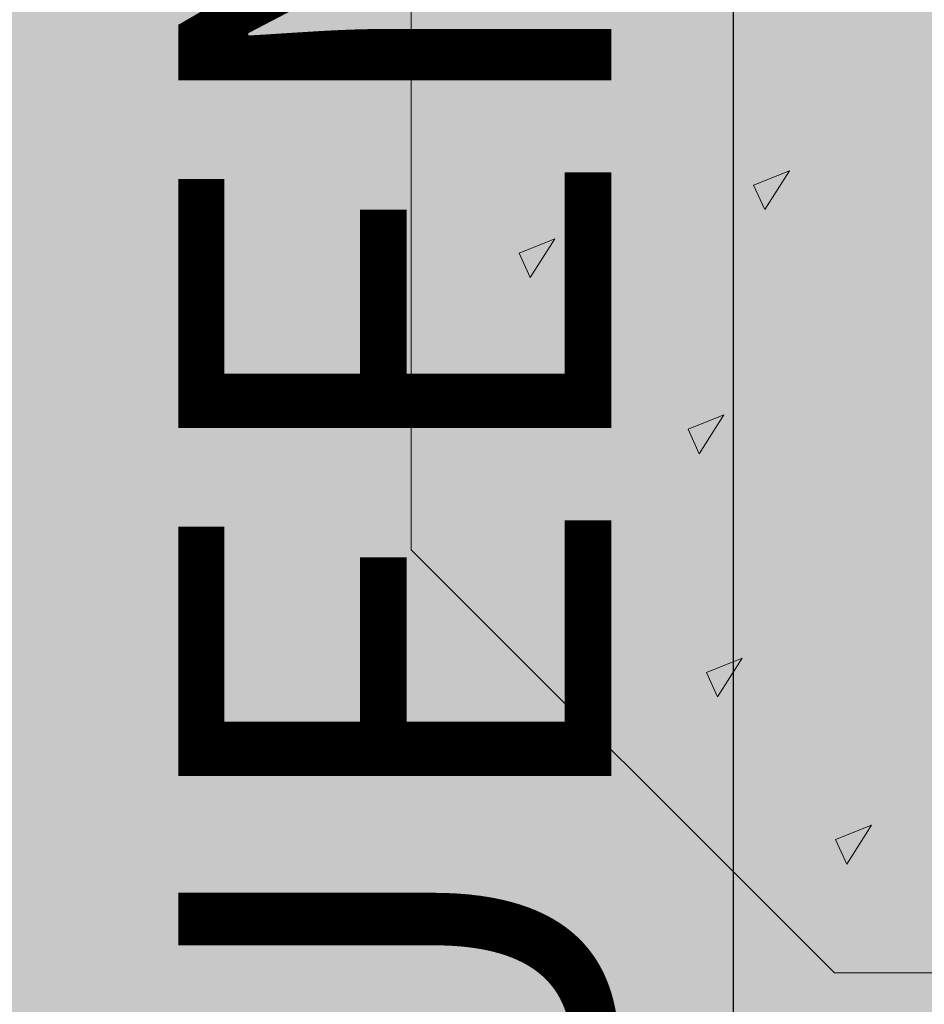
# Model space of a CAD drawing. Units: inches. Extents: x 459864 to 460310, y 324185 to 324787.
# Tile 46 of 112: x 460127.39 to 460139.92, y 324211.25 to 324224.9. Entities that reach past the tile are written whole.
import ezdxf

# ---------------------------------------------------------------- set-up
doc = ezdxf.new("R2010")
doc.units = ezdxf.units.IN
for name, color, linetype, lineweight in [('A-ANNO-DIMS', 2, 'Continuous', 18), ('L-HRDS', 9, 'Continuous', 18), ('L-SITE-PATT', 252, 'Continuous', 13)]:
    doc.layers.add(name, color=color, linetype=linetype, lineweight=lineweight)
doc.styles.get("Standard").update_dxf_attribs({"font": 'arial.ttf'})
doc.dimstyles.new('ISO-25', dxfattribs={"dimtxt": 6, "dimasz": 2.5, "dimexe": 1.25, "dimexo": 0.625, "dimtad": 1, "dimdec": 1, "dimlunit": 3, "dimtxsty": 'Standard', "dimcen": 2.5, "dimadec": 0, "dimazin": 0, "dimtfac": 1, "dimtdec": 1, "dimtmove": 0, "dimatfit": 3, "dimfxl": 1, "dimarcsym": 0})

# ---------------------------------------------------------------- blocks, each defined once
blk = doc.blocks.new('Stepping Stone - hexagonal')
for p, q in [((-10.964, 4.202), (-10.964, -4.092)), ((-5.724, 1.164), (-6.221, 0.965)), ((-6.066, 0.626), (-5.724, 1.164)), ((-6.221, 0.965), (-6.066, 0.626)), ((-8.972, 0.221), (-9.469, 0.023)), ((-9.314, -0.317), (-8.972, 0.221)), ((-9.469, 0.023), (-9.314, -0.317)), ((-6.63, -2.222), (-7.127, -2.421)), ((-6.972, -2.76), (-6.63, -2.222)), ((-7.127, -2.421), (-6.972, -2.76)), ((-10.964, -4.092), (-5.099, -9.957)), ((-6.377, -5.594), (-6.874, -5.792)), ((-6.719, -6.132), (-6.377, -5.594)), ((-6.874, -5.792), (-6.719, -6.132)), ((-4.588, -7.91), (-5.085, -8.109)), ((-4.93, -8.448), (-4.588, -7.91)), ((-5.085, -8.109), (-4.93, -8.448)), ((-5.099, -9.957), (3.195, -9.957))]:
    blk.add_line(p, q)
blk = doc.blocks.new('*D28')
at = {"layer": 'A-ANNO-DIMS', "color": 0, "lineweight": -2, "transparency": 16777216}
for p, q in [((460148.65, 324370.7), (460136.025, 324370.7)), ((460137.275, 324368.2), (460137.275, 324293.2)), ((460148.65, 324290.7), (460136.025, 324290.7)), ((460137.275, 324290.7), (460137.275, 324198.69))]:
    blk.add_line(p, q, dxfattribs=at)
at = {"layer": 'A-ANNO-DIMS', "color": 0, "transparency": 16777216}
for points in [[(460136.858, 324368.2), (460137.692, 324368.2), (460137.275, 324370.7)], [(460136.858, 324293.2), (460137.692, 324293.2), (460137.275, 324290.7)]]:
    blk.add_solid(points, dxfattribs=at)
at = {"layer": 'Defpoints', "color": 0, "transparency": 16777216}
for p in [(460149.275, 324370.7), (460137.275, 324290.7), (460149.275, 324290.7)]:
    blk.add_point(p, dxfattribs=at)
at = {"layer": 'A-ANNO-DIMS', "color": 0, "transparency": 16777216, "insert": (460133.363, 324243.445), "char_height": 6, "attachment_point": 5, "rotation": 90}
blk.add_mtext('QUEEN BED 6\'-8" TYP.', dxfattribs=at)
blk = doc.blocks.new('*D34')
at = {"layer": 'A-ANNO-DIMS', "color": 0, "lineweight": -2, "transparency": 16777216}
for p, q in [((460132.814, 324211.063), (460132.814, 324207.434)), ((460152.838, 324211.063), (460152.838, 324207.434)), ((460135.314, 324208.684), (460150.338, 324208.684)), ((460152.838, 324208.684), (460202.984, 324208.684))]:
    blk.add_line(p, q, dxfattribs=at)
at = {"layer": 'A-ANNO-DIMS', "color": 0, "transparency": 16777216}
for points in [[(460135.314, 324209.101), (460135.314, 324208.268), (460132.814, 324208.684)], [(460150.338, 324209.101), (460150.338, 324208.268), (460152.838, 324208.684)]]:
    blk.add_solid(points, dxfattribs=at)
at = {"layer": 'Defpoints', "color": 0, "transparency": 16777216}
for p in [(460132.814, 324211.688), (460152.838, 324211.688), (460152.838, 324208.684)]:
    blk.add_point(p, dxfattribs=at)
at = {"layer": 'A-ANNO-DIMS', "color": 0, "transparency": 16777216, "insert": (460179.161, 324212.373), "char_height": 6, "attachment_point": 5}
blk.add_mtext('PAVER 1\'-8"', dxfattribs=at)

msp = doc.modelspace()

# ---------------------------------------------------------------- hatches: boundary and pattern name
at = {"layer": 'L-SITE-PATT'}
h = msp.add_hatch(dxfattribs=at)
h.set_pattern_fill('DOTS', color=256)
h.paths.add_polyline_path([(460269.804, 324283.483), (460247.115, 324283.483), (460121.929, 324283.483), (460121.929, 324252.473), (460117.429, 324252.473), (460110.124, 324252.473), (460110.124, 324243.287), (460080.83, 324243.287), (460080.83, 324252.473), (460061.115, 324252.473), (460061.115, 324251.882), (460077.909, 324251.882), (460077.909, 324199.483), (460080.83, 324199.483), (460080.83, 324207.553), (460110.124, 324207.553), (460110.124, 324199.483), (460110.813, 324199.483), (460262.115, 324199.483), (460269.804, 324199.483)], flags=17)
edge = h.paths.add_edge_path(flags=0)
edge.add_ellipse((460222.59, 324263.813), major_axis=(-8.485, 8.485), ratio=1, start_angle=405, end_angle=495, ccw=False)
edge.add_line((460214.821, 324254.66), (460214.832, 324254.666))
edge.add_ellipse((460222.59, 324263.813), major_axis=(-8.485, 8.485), ratio=1, start_angle=405, end_angle=495, ccw=False)
edge.add_line((460210.759, 324261.781), (460210.768, 324261.787))
edge.add_ellipse((460222.59, 324263.813), major_axis=(-8.485, 8.485), ratio=1, start_angle=405, end_angle=495, ccw=False)
edge.add_ellipse((460222.59, 324263.813), major_axis=(-8.485, 8.485), ratio=1, start_angle=392.754, end_angle=405, ccw=False)
edge.add_ellipse((460222.59, 324263.813), major_axis=(-8.485, 8.485), ratio=1, start_angle=380.9347, end_angle=392.754, ccw=False)
edge.add_line((460211.337, 324267.985), (460211.34, 324267.985))
edge.add_ellipse((460222.59, 324263.813), major_axis=(-8.485, 8.485), ratio=1, start_angle=380.9347, end_angle=392.754, ccw=False)
edge.add_ellipse((460222.59, 324263.813), major_axis=(-8.485, 8.485), ratio=1, start_angle=347.9015, end_angle=380.9347, ccw=False)
edge.add_ellipse((460222.59, 324263.813), major_axis=(-8.485, 8.485), ratio=1, start_angle=327.0619, end_angle=347.9015, ccw=False)
edge.add_ellipse((460222.59, 324263.813), major_axis=(-8.485, 8.485), ratio=1, start_angle=278.3246, end_angle=327.0619, ccw=False)
edge.add_line((460225.158, 324275.536), (460225.158, 324275.535))
edge.add_ellipse((460222.59, 324263.813), major_axis=(-8.485, 8.485), ratio=1, start_angle=278.3246, end_angle=327.0619, ccw=False)
edge.add_ellipse((460222.59, 324263.813), major_axis=(-8.485, 8.485), ratio=1, start_angle=260.6436, end_angle=278.3246, ccw=False)
edge.add_ellipse((460222.59, 324263.813), major_axis=(-8.485, 8.485), ratio=1, start_angle=225, end_angle=260.6436, ccw=False)
edge.add_line((460234.509, 324265.243), (460234.501, 324265.239))
edge.add_ellipse((460222.59, 324263.813), major_axis=(-8.485, 8.485), ratio=1, start_angle=225, end_angle=260.6436, ccw=False)
edge.add_ellipse((460222.59, 324263.813), major_axis=(-8.485, 8.485), ratio=1, start_angle=495, end_angle=585, ccw=False)
edge.add_line((460234.437, 324261.861), (460234.424, 324261.858))
edge.add_ellipse((460222.59, 324263.813), major_axis=(-8.485, 8.485), ratio=1, start_angle=495, end_angle=585, ccw=False)
edge.add_line((460227.95, 324253.067), (460227.946, 324253.083))
edge.add_ellipse((460222.59, 324263.813), major_axis=(-8.485, 8.485), ratio=1, start_angle=495, end_angle=585, ccw=False)
edge.add_line((460226.223, 324252.369), (460226.211, 324252.38))
edge.add_ellipse((460222.59, 324263.813), major_axis=(-8.485, 8.485), ratio=1, start_angle=495, end_angle=585, ccw=False)
h.paths.add_polyline_path([(460219.651, 324254.347), (460218.461, 324253.545), (460218.275, 324254.789), (460219.642, 324256.542), (460219.625, 324260.848), (460216.11, 324257.333), (460214.35, 324256.978), (460215.416, 324259.356), (460212.524, 324258.496), (460213.137, 324259.93), (460218.507, 324263.813), (460222.59, 324263.813), (460222.59, 324267.807), (460218.176, 324272.212), (460219.026, 324274.639), (460222.59, 324272.811), (460222.59, 324275.423), (460223.057, 324274.825), (460222.675, 324273.492), (460225.912, 324267.135), (460219.625, 324260.848)], flags=0)
edge = h.paths.add_edge_path(flags=0)
edge.add_ellipse((460194.576, 324264.046), major_axis=(-8.485, 8.485), ratio=1, start_angle=495, end_angle=585, ccw=False)
edge.add_line((460199.936, 324253.3), (460199.932, 324253.316))
edge.add_ellipse((460194.576, 324264.046), major_axis=(-8.485, 8.485), ratio=1, start_angle=495, end_angle=585, ccw=False)
edge.add_line((460198.208, 324252.603), (460198.196, 324252.613))
edge.add_ellipse((460194.576, 324264.046), major_axis=(-8.485, 8.485), ratio=1, start_angle=495, end_angle=585, ccw=False)
edge.add_ellipse((460194.576, 324264.046), major_axis=(-8.485, 8.485), ratio=1, start_angle=405, end_angle=495, ccw=False)
edge.add_line((460186.806, 324254.893), (460186.817, 324254.899))
edge.add_ellipse((460194.576, 324264.046), major_axis=(-8.485, 8.485), ratio=1, start_angle=405, end_angle=495, ccw=False)
edge.add_line((460182.744, 324262.014), (460182.753, 324262.02))
edge.add_ellipse((460194.576, 324264.046), major_axis=(-8.485, 8.485), ratio=1, start_angle=405, end_angle=495, ccw=False)
edge.add_ellipse((460194.576, 324264.046), major_axis=(-8.485, 8.485), ratio=1, start_angle=392.754, end_angle=405, ccw=False)
edge.add_ellipse((460194.576, 324264.046), major_axis=(-8.485, 8.485), ratio=1, start_angle=380.9347, end_angle=392.754, ccw=False)
edge.add_line((460183.323, 324268.218), (460183.326, 324268.218))
edge.add_ellipse((460194.576, 324264.046), major_axis=(-8.485, 8.485), ratio=1, start_angle=380.9347, end_angle=392.754, ccw=False)
edge.add_ellipse((460194.576, 324264.046), major_axis=(-8.485, 8.485), ratio=1, start_angle=347.9015, end_angle=380.9347, ccw=False)
edge.add_ellipse((460194.576, 324264.046), major_axis=(-8.485, 8.485), ratio=1, start_angle=327.0619, end_angle=347.9015, ccw=False)
edge.add_ellipse((460194.576, 324264.046), major_axis=(-8.485, 8.485), ratio=1, start_angle=278.3246, end_angle=327.0619, ccw=False)
edge.add_line((460197.144, 324275.769), (460197.143, 324275.768))
edge.add_ellipse((460194.576, 324264.046), major_axis=(-8.485, 8.485), ratio=1, start_angle=278.3246, end_angle=327.0619, ccw=False)
edge.add_ellipse((460194.576, 324264.046), major_axis=(-8.485, 8.485), ratio=1, start_angle=260.6436, end_angle=278.3246, ccw=False)
edge.add_ellipse((460194.576, 324264.046), major_axis=(-8.485, 8.485), ratio=1, start_angle=225, end_angle=260.6436, ccw=False)
edge.add_line((460206.494, 324265.476), (460206.487, 324265.473))
edge.add_ellipse((460194.576, 324264.046), major_axis=(-8.485, 8.485), ratio=1, start_angle=225, end_angle=260.6436, ccw=False)
edge.add_ellipse((460194.576, 324264.046), major_axis=(-8.485, 8.485), ratio=1, start_angle=495, end_angle=585, ccw=False)
edge.add_line((460206.422, 324262.094), (460206.409, 324262.091))
h.paths.add_polyline_path([(460191.61, 324261.081), (460191.637, 324254.58), (460190.447, 324253.778), (460190.261, 324255.023), (460191.628, 324256.775), (460191.61, 324261.081), (460188.096, 324257.566), (460186.335, 324257.211), (460187.402, 324259.589), (460184.509, 324258.729), (460185.123, 324260.163), (460190.493, 324264.046), (460194.576, 324264.046), (460194.576, 324268.04), (460190.161, 324272.446), (460191.011, 324274.872), (460194.576, 324273.044), (460194.576, 324275.657), (460195.043, 324275.058), (460194.661, 324273.725), (460197.897, 324267.368)], flags=0)
edge = h.paths.add_edge_path(flags=0)
edge.add_ellipse((460252.912, 324263.578), major_axis=(-8.485, 8.485), ratio=1, start_angle=405, end_angle=495, ccw=False)
edge.add_line((460241.081, 324261.545), (460241.089, 324261.551))
edge.add_ellipse((460252.912, 324263.578), major_axis=(-8.485, 8.485), ratio=1, start_angle=405, end_angle=495, ccw=False)
edge.add_ellipse((460252.912, 324263.578), major_axis=(-8.485, 8.485), ratio=1, start_angle=392.754, end_angle=405, ccw=False)
edge.add_ellipse((460252.912, 324263.578), major_axis=(-8.485, 8.485), ratio=1, start_angle=380.9347, end_angle=392.754, ccw=False)
edge.add_line((460241.659, 324267.749), (460241.662, 324267.749))
edge.add_ellipse((460252.912, 324263.578), major_axis=(-8.485, 8.485), ratio=1, start_angle=380.9347, end_angle=392.754, ccw=False)
edge.add_ellipse((460252.912, 324263.578), major_axis=(-8.485, 8.485), ratio=1, start_angle=347.9015, end_angle=380.9347, ccw=False)
edge.add_ellipse((460252.912, 324263.578), major_axis=(-8.485, 8.485), ratio=1, start_angle=327.0619, end_angle=347.9015, ccw=False)
edge.add_ellipse((460252.912, 324263.578), major_axis=(-8.485, 8.485), ratio=1, start_angle=278.3246, end_angle=327.0619, ccw=False)
edge.add_line((460255.48, 324275.3), (460255.479, 324275.299))
edge.add_ellipse((460252.912, 324263.578), major_axis=(-8.485, 8.485), ratio=1, start_angle=278.3246, end_angle=327.0619, ccw=False)
edge.add_ellipse((460252.912, 324263.578), major_axis=(-8.485, 8.485), ratio=1, start_angle=260.6436, end_angle=278.3246, ccw=False)
edge.add_ellipse((460252.912, 324263.578), major_axis=(-8.485, 8.485), ratio=1, start_angle=225, end_angle=260.6436, ccw=False)
edge.add_line((460264.83, 324265.007), (460264.823, 324265.004))
edge.add_ellipse((460252.912, 324263.578), major_axis=(-8.485, 8.485), ratio=1, start_angle=225, end_angle=260.6436, ccw=False)
edge.add_ellipse((460252.912, 324263.578), major_axis=(-8.485, 8.485), ratio=1, start_angle=495, end_angle=585, ccw=False)
edge.add_line((460264.758, 324261.626), (460264.745, 324261.622))
edge.add_ellipse((460252.912, 324263.578), major_axis=(-8.485, 8.485), ratio=1, start_angle=495, end_angle=585, ccw=False)
edge.add_line((460258.272, 324252.832), (460258.268, 324252.848))
edge.add_ellipse((460252.912, 324263.578), major_axis=(-8.485, 8.485), ratio=1, start_angle=495, end_angle=585, ccw=False)
edge.add_line((460256.545, 324252.134), (460256.533, 324252.144))
edge.add_ellipse((460252.912, 324263.578), major_axis=(-8.485, 8.485), ratio=1, start_angle=495, end_angle=585, ccw=False)
edge.add_ellipse((460252.912, 324263.578), major_axis=(-8.485, 8.485), ratio=1, start_angle=405, end_angle=495, ccw=False)
edge.add_line((460245.143, 324254.424), (460245.153, 324254.43))
h.paths.add_polyline_path([(460244.672, 324256.742), (460245.738, 324259.12), (460242.846, 324258.26), (460243.459, 324259.694), (460248.829, 324263.578), (460252.912, 324263.578), (460252.912, 324267.571), (460248.497, 324271.977), (460249.348, 324274.403), (460252.912, 324272.576), (460252.912, 324275.188), (460253.379, 324274.589), (460252.997, 324273.257), (460256.233, 324266.899), (460249.946, 324260.612), (460249.973, 324254.111), (460248.783, 324253.309), (460248.597, 324254.554), (460249.964, 324256.306), (460249.946, 324260.612), (460246.432, 324257.097)], flags=0)
edge = h.paths.add_edge_path(flags=0)
edge.add_ellipse((460167.439, 324262.833), major_axis=(-8.485, 8.485), ratio=1, start_angle=495, end_angle=585, ccw=False)
edge.add_line((460172.799, 324252.087), (460172.795, 324252.103))
edge.add_ellipse((460167.439, 324262.833), major_axis=(-8.485, 8.485), ratio=1, start_angle=495, end_angle=585, ccw=False)
edge.add_line((460171.071, 324251.389), (460171.059, 324251.399))
edge.add_ellipse((460167.439, 324262.833), major_axis=(-8.485, 8.485), ratio=1, start_angle=495, end_angle=585, ccw=False)
edge.add_ellipse((460167.439, 324262.833), major_axis=(-8.485, 8.485), ratio=1, start_angle=405, end_angle=495, ccw=False)
edge.add_line((460159.669, 324253.679), (460159.68, 324253.685))
edge.add_ellipse((460167.439, 324262.833), major_axis=(-8.485, 8.485), ratio=1, start_angle=405, end_angle=495, ccw=False)
edge.add_line((460155.607, 324260.8), (460155.616, 324260.806))
edge.add_ellipse((460167.439, 324262.833), major_axis=(-8.485, 8.485), ratio=1, start_angle=405, end_angle=495, ccw=False)
edge.add_ellipse((460167.439, 324262.833), major_axis=(-8.485, 8.485), ratio=1, start_angle=392.754, end_angle=405, ccw=False)
edge.add_ellipse((460167.439, 324262.833), major_axis=(-8.485, 8.485), ratio=1, start_angle=380.9347, end_angle=392.754, ccw=False)
edge.add_line((460156.185, 324267.005), (460156.189, 324267.005))
edge.add_ellipse((460167.439, 324262.833), major_axis=(-8.485, 8.485), ratio=1, start_angle=380.9347, end_angle=392.754, ccw=False)
edge.add_ellipse((460167.439, 324262.833), major_axis=(-8.485, 8.485), ratio=1, start_angle=347.9015, end_angle=380.9347, ccw=False)
edge.add_ellipse((460167.439, 324262.833), major_axis=(-8.485, 8.485), ratio=1, start_angle=327.0619, end_angle=347.9015, ccw=False)
edge.add_ellipse((460167.439, 324262.833), major_axis=(-8.485, 8.485), ratio=1, start_angle=278.3246, end_angle=327.0619, ccw=False)
edge.add_line((460170.007, 324274.556), (460170.006, 324274.554))
edge.add_ellipse((460167.439, 324262.833), major_axis=(-8.485, 8.485), ratio=1, start_angle=278.3246, end_angle=327.0619, ccw=False)
edge.add_ellipse((460167.439, 324262.833), major_axis=(-8.485, 8.485), ratio=1, start_angle=260.6436, end_angle=278.3246, ccw=False)
edge.add_ellipse((460167.439, 324262.833), major_axis=(-8.485, 8.485), ratio=1, start_angle=225, end_angle=260.6436, ccw=False)
edge.add_line((460179.357, 324264.262), (460179.35, 324264.259))
edge.add_ellipse((460167.439, 324262.833), major_axis=(-8.485, 8.485), ratio=1, start_angle=225, end_angle=260.6436, ccw=False)
edge.add_ellipse((460167.439, 324262.833), major_axis=(-8.485, 8.485), ratio=1, start_angle=495, end_angle=585, ccw=False)
edge.add_line((460179.285, 324260.881), (460179.272, 324260.877))
h.paths.add_polyline_path([(460164.473, 324259.867), (460164.5, 324253.366), (460163.31, 324252.565), (460163.124, 324253.809), (460164.491, 324255.561), (460164.473, 324259.867), (460160.958, 324256.353), (460159.198, 324255.998), (460160.265, 324258.375), (460157.372, 324257.515), (460157.986, 324258.949), (460163.356, 324262.833), (460167.439, 324262.833), (460167.439, 324266.826), (460163.024, 324271.232), (460163.874, 324273.659), (460167.439, 324271.831), (460167.439, 324274.443), (460167.905, 324273.844), (460167.524, 324272.512), (460170.76, 324266.154)], flags=0)
edge = h.paths.add_edge_path(flags=0)
edge.add_ellipse((460140.758, 324262.37), major_axis=(-8.485, 8.485), ratio=1, start_angle=495, end_angle=585, ccw=False)
edge.add_line((460146.118, 324251.624), (460146.114, 324251.639))
edge.add_ellipse((460140.758, 324262.37), major_axis=(-8.485, 8.485), ratio=1, start_angle=495, end_angle=585, ccw=False)
edge.add_line((460144.391, 324250.926), (460144.379, 324250.936))
edge.add_ellipse((460140.758, 324262.37), major_axis=(-8.485, 8.485), ratio=1, start_angle=495, end_angle=585, ccw=False)
edge.add_ellipse((460140.758, 324262.37), major_axis=(-8.485, 8.485), ratio=1, start_angle=405, end_angle=495, ccw=False)
edge.add_line((460132.989, 324253.216), (460132.999, 324253.222))
edge.add_ellipse((460140.758, 324262.37), major_axis=(-8.485, 8.485), ratio=1, start_angle=405, end_angle=495, ccw=False)
edge.add_line((460128.927, 324260.337), (460128.935, 324260.343))
edge.add_ellipse((460140.758, 324262.37), major_axis=(-8.485, 8.485), ratio=1, start_angle=405, end_angle=495, ccw=False)
edge.add_ellipse((460140.758, 324262.37), major_axis=(-8.485, 8.485), ratio=1, start_angle=392.754, end_angle=405, ccw=False)
edge.add_ellipse((460140.758, 324262.37), major_axis=(-8.485, 8.485), ratio=1, start_angle=380.9347, end_angle=392.754, ccw=False)
edge.add_line((460129.505, 324266.541), (460129.508, 324266.541))
edge.add_ellipse((460140.758, 324262.37), major_axis=(-8.485, 8.485), ratio=1, start_angle=380.9347, end_angle=392.754, ccw=False)
edge.add_ellipse((460140.758, 324262.37), major_axis=(-8.485, 8.485), ratio=1, start_angle=347.9015, end_angle=380.9347, ccw=False)
edge.add_ellipse((460140.758, 324262.37), major_axis=(-8.485, 8.485), ratio=1, start_angle=327.0619, end_angle=347.9015, ccw=False)
edge.add_ellipse((460140.758, 324262.37), major_axis=(-8.485, 8.485), ratio=1, start_angle=278.3246, end_angle=327.0619, ccw=False)
edge.add_line((460143.326, 324274.092), (460143.325, 324274.091))
edge.add_ellipse((460140.758, 324262.37), major_axis=(-8.485, 8.485), ratio=1, start_angle=278.3246, end_angle=327.0619, ccw=False)
edge.add_ellipse((460140.758, 324262.37), major_axis=(-8.485, 8.485), ratio=1, start_angle=260.6436, end_angle=278.3246, ccw=False)
edge.add_ellipse((460140.758, 324262.37), major_axis=(-8.485, 8.485), ratio=1, start_angle=225, end_angle=260.6436, ccw=False)
edge.add_line((460152.677, 324263.799), (460152.669, 324263.796))
edge.add_ellipse((460140.758, 324262.37), major_axis=(-8.485, 8.485), ratio=1, start_angle=225, end_angle=260.6436, ccw=False)
edge.add_ellipse((460140.758, 324262.37), major_axis=(-8.485, 8.485), ratio=1, start_angle=495, end_angle=585, ccw=False)
edge.add_line((460152.604, 324260.418), (460152.592, 324260.414))
h.paths.add_polyline_path([(460137.792, 324259.404), (460137.819, 324252.903), (460136.629, 324252.101), (460136.443, 324253.346), (460137.81, 324255.098), (460137.792, 324259.404), (460134.278, 324255.889), (460132.518, 324255.534), (460133.584, 324257.912), (460130.692, 324257.052), (460131.305, 324258.486), (460136.675, 324262.37), (460140.758, 324262.37), (460140.758, 324266.363), (460136.343, 324270.769), (460137.194, 324273.195), (460140.758, 324271.367), (460140.758, 324273.98), (460141.225, 324273.381), (460140.843, 324272.049), (460144.079, 324265.691)], flags=0)
h.paths.add_polyline_path([(460110.124, 324227.414), (460080.83, 324227.414), (460080.83, 324235.484), (460110.124, 324235.484)], flags=16)
h.paths.add_polyline_path([(460110.124, 324220.797), (460110.124, 324212.727), (460080.83, 324212.727), (460080.83, 324220.797)], flags=16)
h.paths.add_polyline_path([(460269.804, 324283.483), (460247.115, 324283.483), (460121.929, 324283.483), (460121.929, 324252.473), (460117.429, 324252.473), (460110.124, 324252.473), (460110.124, 324243.287), (460080.83, 324243.287), (460080.83, 324252.473), (460061.115, 324252.473), (460061.115, 324251.882), (460077.909, 324251.882), (460077.909, 324199.483), (460080.83, 324199.483), (460080.83, 324207.553), (460110.124, 324207.553), (460110.124, 324199.483), (460262.115, 324199.483), (460269.804, 324199.483)], flags=17)
h.paths.add_polyline_path([(460219.651, 324254.347), (460218.461, 324253.545), (460218.275, 324254.789), (460219.642, 324256.542), (460219.625, 324260.848), (460216.11, 324257.333), (460214.35, 324256.978), (460215.416, 324259.356), (460212.524, 324258.496), (460213.137, 324259.93), (460218.507, 324263.813), (460222.59, 324263.813), (460220.18, 324266.223), (460215.461, 324265.308), (460211.835, 324266.137), (460216.247, 324267.985), (460218.418, 324267.985), (460222.59, 324263.813), (460222.59, 324267.807), (460218.176, 324272.212), (460219.026, 324274.639), (460222.59, 324272.811), (460222.59, 324275.423), (460223.057, 324274.825), (460222.675, 324273.492), (460225.912, 324267.135), (460222.59, 324263.813), (460231.383, 324263.813), (460228.485, 324262.488), (460224.425, 324261.978), (460228.68, 324257.724), (460228.966, 324254.791), (460227.142, 324256.537), (460227.542, 324254.819), (460227.333, 324253.614), (460222.59, 324259.985), (460222.59, 324255.497), (460221.377, 324256.541), (460220.576, 324261.799), (460219.625, 324260.848)], flags=0)
h.paths.add_polyline_path([(460199.127, 324256.77), (460199.528, 324255.052), (460199.319, 324253.848), (460194.576, 324260.218), (460194.576, 324255.73), (460193.363, 324256.774), (460192.561, 324262.032), (460191.61, 324261.081), (460191.637, 324254.58), (460190.447, 324253.778), (460190.261, 324255.023), (460191.628, 324256.775), (460191.61, 324261.081), (460188.096, 324257.566), (460186.335, 324257.211), (460187.402, 324259.589), (460184.509, 324258.729), (460185.123, 324260.163), (460190.493, 324264.046), (460194.576, 324264.046), (460192.166, 324266.456), (460187.446, 324265.541), (460183.82, 324266.37), (460188.232, 324268.218), (460190.404, 324268.218), (460194.576, 324264.046), (460194.576, 324268.04), (460190.161, 324272.446), (460191.011, 324274.872), (460194.576, 324273.044), (460194.576, 324275.657), (460195.043, 324275.058), (460194.661, 324273.725), (460197.897, 324267.368), (460194.576, 324264.046), (460203.368, 324264.046), (460200.47, 324262.721), (460196.411, 324262.212), (460200.665, 324257.957), (460200.951, 324255.024)], flags=0)
h.paths.add_polyline_path([(460244.672, 324256.742), (460245.738, 324259.12), (460242.846, 324258.26), (460243.459, 324259.694), (460248.829, 324263.578), (460252.912, 324263.578), (460250.502, 324265.987), (460245.783, 324265.072), (460242.156, 324265.901), (460246.568, 324267.749), (460248.74, 324267.749), (460252.912, 324263.578), (460252.912, 324267.571), (460248.497, 324271.977), (460249.348, 324274.403), (460252.912, 324272.576), (460252.912, 324275.188), (460253.379, 324274.589), (460252.997, 324273.257), (460256.233, 324266.899), (460252.912, 324263.578), (460261.705, 324263.578), (460258.806, 324262.252), (460254.747, 324261.743), (460259.002, 324257.488), (460259.288, 324254.555), (460257.463, 324256.301), (460257.864, 324254.583), (460257.655, 324253.379), (460252.912, 324259.749), (460252.912, 324255.261), (460251.699, 324256.305), (460250.897, 324261.563), (460249.946, 324260.612), (460249.973, 324254.111), (460248.783, 324253.309), (460248.597, 324254.554), (460249.964, 324256.306), (460249.946, 324260.612), (460246.432, 324257.097)], flags=0)
h.paths.add_polyline_path([(460173.528, 324256.743), (460173.814, 324253.811), (460171.99, 324255.556), (460172.39, 324253.838), (460172.182, 324252.634), (460167.439, 324259.004), (460167.439, 324254.516), (460166.226, 324255.56), (460165.424, 324260.818), (460164.473, 324259.867), (460164.5, 324253.366), (460163.31, 324252.565), (460163.124, 324253.809), (460164.491, 324255.561), (460164.473, 324259.867), (460160.958, 324256.353), (460159.198, 324255.998), (460160.265, 324258.375), (460157.372, 324257.515), (460157.986, 324258.949), (460163.356, 324262.833), (460167.439, 324262.833), (460165.029, 324265.243), (460160.309, 324264.327), (460156.683, 324265.156), (460161.095, 324267.005), (460163.267, 324267.005), (460167.439, 324262.833), (460167.439, 324266.826), (460163.024, 324271.232), (460163.874, 324273.659), (460167.439, 324271.831), (460167.439, 324274.443), (460167.905, 324273.844), (460167.524, 324272.512), (460170.76, 324266.154), (460167.439, 324262.833), (460176.231, 324262.833), (460173.333, 324261.507), (460169.274, 324260.998)], flags=0)
h.paths.add_polyline_path([(460146.848, 324256.28), (460147.134, 324253.347), (460145.31, 324255.093), (460145.71, 324253.375), (460145.501, 324252.171), (460140.758, 324258.541), (460140.758, 324254.053), (460139.545, 324255.097), (460138.744, 324260.355), (460137.792, 324259.404), (460137.819, 324252.903), (460136.629, 324252.101), (460136.443, 324253.346), (460137.81, 324255.098), (460137.792, 324259.404), (460134.278, 324255.889), (460132.518, 324255.534), (460133.584, 324257.912), (460130.692, 324257.052), (460131.305, 324258.486), (460136.675, 324262.37), (460140.758, 324262.37), (460138.348, 324264.779), (460133.629, 324263.864), (460130.002, 324264.693), (460134.414, 324266.541), (460136.586, 324266.541), (460140.758, 324262.37), (460140.758, 324266.363), (460136.343, 324270.769), (460137.194, 324273.195), (460140.758, 324271.367), (460140.758, 324273.98), (460141.225, 324273.381), (460140.843, 324272.049), (460144.079, 324265.691), (460140.758, 324262.37), (460149.551, 324262.37), (460146.653, 324261.044), (460142.593, 324260.535)], flags=0)
edge = h.paths.add_edge_path()
edge.add_line((460269.804, 324272.549), (460260.881, 324272.549))
edge.add_ellipse((460252.912, 324263.578), major_axis=(-8.485, 8.485), ratio=1, start_angle=260.6436, end_angle=273.3846, ccw=False)
edge.add_line((460262.283, 324271.092), (460262.261, 324271.091))
edge.add_ellipse((460252.912, 324263.578), major_axis=(-8.485, 8.485), ratio=1, start_angle=260.6436, end_angle=273.3846, ccw=False)
edge.add_ellipse((460252.912, 324263.578), major_axis=(-8.485, 8.485), ratio=1, start_angle=225, end_angle=260.6436, ccw=False)
edge.add_line((460263.609, 324269.063), (460263.572, 324269.058))
edge.add_ellipse((460252.912, 324263.578), major_axis=(-8.485, 8.485), ratio=1, start_angle=225, end_angle=260.6436, ccw=False)
edge.add_line((460264.615, 324266.306), (460264.585, 324266.305))
edge.add_ellipse((460252.912, 324263.578), major_axis=(-8.485, 8.485), ratio=1, start_angle=225, end_angle=260.6436, ccw=False)
edge.add_line((460264.83, 324265.007), (460264.823, 324265.004))
edge.add_ellipse((460252.912, 324263.578), major_axis=(-8.485, 8.485), ratio=1, start_angle=225, end_angle=260.6436, ccw=False)
edge.add_ellipse((460252.912, 324263.578), major_axis=(-8.485, 8.485), ratio=1, start_angle=495, end_angle=585, ccw=False)
edge.add_line((460264.758, 324261.626), (460264.745, 324261.622))
edge.add_ellipse((460252.912, 324263.578), major_axis=(-8.485, 8.485), ratio=1, start_angle=495, end_angle=585, ccw=False)
edge.add_line((460263.442, 324257.739), (460263.389, 324257.779))
edge.add_ellipse((460252.912, 324263.578), major_axis=(-8.485, 8.485), ratio=1, start_angle=495, end_angle=585, ccw=False)
edge.add_line((460258.128, 324252.744), (460258.102, 324252.779))
edge.add_ellipse((460252.912, 324263.578), major_axis=(-8.485, 8.485), ratio=1, start_angle=495, end_angle=585, ccw=False)
edge.add_line((460256.545, 324252.134), (460256.533, 324252.144))
edge.add_ellipse((460252.912, 324263.578), major_axis=(-8.485, 8.485), ratio=1, start_angle=495, end_angle=585, ccw=False)
edge.add_ellipse((460252.912, 324263.578), major_axis=(-8.485, 8.485), ratio=1, start_angle=405, end_angle=495, ccw=False)
edge.add_line((460250.594, 324251.78), (460250.605, 324251.82))
edge.add_ellipse((460252.912, 324263.578), major_axis=(-8.485, 8.485), ratio=1, start_angle=405, end_angle=495, ccw=False)
edge.add_line((460245.143, 324254.424), (460245.153, 324254.43))
edge.add_ellipse((460252.912, 324263.578), major_axis=(-8.485, 8.485), ratio=1, start_angle=405, end_angle=495, ccw=False)
edge.add_line((460243.525, 324256.059), (460243.56, 324256.091))
edge.add_ellipse((460252.912, 324263.578), major_axis=(-8.485, 8.485), ratio=1, start_angle=405, end_angle=495, ccw=False)
edge.add_line((460241.44, 324259.893), (460241.522, 324259.896))
edge.add_ellipse((460252.912, 324263.578), major_axis=(-8.485, 8.485), ratio=1, start_angle=405, end_angle=495, ccw=False)
edge.add_line((460241.081, 324261.545), (460241.089, 324261.551))
edge.add_ellipse((460252.912, 324263.578), major_axis=(-8.485, 8.485), ratio=1, start_angle=405, end_angle=495, ccw=False)
edge.add_ellipse((460252.912, 324263.578), major_axis=(-8.485, 8.485), ratio=1, start_angle=392.754, end_angle=405, ccw=False)
edge.add_line((460241.05, 324265.438), (460241.063, 324265.443))
edge.add_ellipse((460252.912, 324263.578), major_axis=(-8.485, 8.485), ratio=1, start_angle=392.754, end_angle=405, ccw=False)
edge.add_ellipse((460252.912, 324263.578), major_axis=(-8.485, 8.485), ratio=1, start_angle=380.9347, end_angle=392.754, ccw=False)
edge.add_line((460241.452, 324267.176), (460241.469, 324267.171))
edge.add_ellipse((460252.912, 324263.578), major_axis=(-8.485, 8.485), ratio=1, start_angle=380.9347, end_angle=392.754, ccw=False)
edge.add_line((460241.659, 324267.749), (460241.662, 324267.749))
edge.add_ellipse((460252.912, 324263.578), major_axis=(-8.485, 8.485), ratio=1, start_angle=380.9347, end_angle=392.754, ccw=False)
edge.add_ellipse((460252.912, 324263.578), major_axis=(-8.485, 8.485), ratio=1, start_angle=356.6154, end_angle=380.9347, ccw=False)
edge.add_line((460244.88, 324272.488), (460244.713, 324272.549))
edge.add_line((460244.713, 324272.549), (460230.817, 324272.549))
edge.add_ellipse((460222.59, 324263.813), major_axis=(-8.485, 8.485), ratio=1, start_angle=260.6436, end_angle=271.7178, ccw=False)
edge.add_ellipse((460222.59, 324263.813), major_axis=(-8.485, 8.485), ratio=1, start_angle=225, end_angle=260.6436, ccw=False)
edge.add_line((460233.287, 324269.299), (460233.25, 324269.294))
edge.add_ellipse((460222.59, 324263.813), major_axis=(-8.485, 8.485), ratio=1, start_angle=225, end_angle=260.6436, ccw=False)
edge.add_line((460234.294, 324266.541), (460234.264, 324266.541))
edge.add_ellipse((460222.59, 324263.813), major_axis=(-8.485, 8.485), ratio=1, start_angle=225, end_angle=260.6436, ccw=False)
edge.add_line((460234.509, 324265.243), (460234.501, 324265.239))
edge.add_ellipse((460222.59, 324263.813), major_axis=(-8.485, 8.485), ratio=1, start_angle=225, end_angle=260.6436, ccw=False)
edge.add_ellipse((460222.59, 324263.813), major_axis=(-8.485, 8.485), ratio=1, start_angle=495, end_angle=585, ccw=False)
edge.add_line((460234.437, 324261.861), (460234.424, 324261.858))
edge.add_ellipse((460222.59, 324263.813), major_axis=(-8.485, 8.485), ratio=1, start_angle=495, end_angle=585, ccw=False)
edge.add_line((460233.121, 324257.975), (460233.068, 324258.015))
edge.add_ellipse((460222.59, 324263.813), major_axis=(-8.485, 8.485), ratio=1, start_angle=495, end_angle=585, ccw=False)
edge.add_line((460227.806, 324252.979), (460227.78, 324253.014))
edge.add_ellipse((460222.59, 324263.813), major_axis=(-8.485, 8.485), ratio=1, start_angle=495, end_angle=585, ccw=False)
edge.add_line((460226.223, 324252.369), (460226.211, 324252.38))
edge.add_ellipse((460222.59, 324263.813), major_axis=(-8.485, 8.485), ratio=1, start_angle=495, end_angle=585, ccw=False)
edge.add_ellipse((460222.59, 324263.813), major_axis=(-8.485, 8.485), ratio=1, start_angle=405, end_angle=495, ccw=False)
edge.add_line((460220.272, 324252.016), (460220.283, 324252.055))
edge.add_ellipse((460222.59, 324263.813), major_axis=(-8.485, 8.485), ratio=1, start_angle=405, end_angle=495, ccw=False)
edge.add_line((460214.821, 324254.66), (460214.832, 324254.666))
edge.add_ellipse((460222.59, 324263.813), major_axis=(-8.485, 8.485), ratio=1, start_angle=405, end_angle=495, ccw=False)
edge.add_line((460213.203, 324256.295), (460213.239, 324256.327))
edge.add_ellipse((460222.59, 324263.813), major_axis=(-8.485, 8.485), ratio=1, start_angle=405, end_angle=495, ccw=False)
edge.add_line((460211.118, 324260.128), (460211.201, 324260.131))
edge.add_ellipse((460222.59, 324263.813), major_axis=(-8.485, 8.485), ratio=1, start_angle=405, end_angle=495, ccw=False)
edge.add_line((460210.759, 324261.781), (460210.768, 324261.787))
edge.add_ellipse((460222.59, 324263.813), major_axis=(-8.485, 8.485), ratio=1, start_angle=405, end_angle=495, ccw=False)
edge.add_ellipse((460222.59, 324263.813), major_axis=(-8.485, 8.485), ratio=1, start_angle=392.754, end_angle=405, ccw=False)
edge.add_line((460210.729, 324265.673), (460210.741, 324265.678))
edge.add_ellipse((460222.59, 324263.813), major_axis=(-8.485, 8.485), ratio=1, start_angle=392.754, end_angle=405, ccw=False)
edge.add_ellipse((460222.59, 324263.813), major_axis=(-8.485, 8.485), ratio=1, start_angle=380.9347, end_angle=392.754, ccw=False)
edge.add_line((460211.13, 324267.412), (460211.147, 324267.407))
edge.add_ellipse((460222.59, 324263.813), major_axis=(-8.485, 8.485), ratio=1, start_angle=380.9347, end_angle=392.754, ccw=False)
edge.add_line((460211.337, 324267.985), (460211.34, 324267.985))
edge.add_ellipse((460222.59, 324263.813), major_axis=(-8.485, 8.485), ratio=1, start_angle=380.9347, end_angle=392.754, ccw=False)
edge.add_ellipse((460222.59, 324263.813), major_axis=(-8.485, 8.485), ratio=1, start_angle=358.2822, end_angle=380.9347, ccw=False)
edge.add_line((460213.705, 324271.902), (460213.709, 324271.869))
edge.add_ellipse((460222.59, 324263.813), major_axis=(-8.485, 8.485), ratio=1, start_angle=358.2822, end_angle=380.9347, ccw=False)
edge.add_line((460214.363, 324272.549), (460203.078, 324272.549))
edge.add_line((460203.078, 324272.549), (460203.06, 324272.531))
edge.add_ellipse((460194.576, 324264.046), major_axis=(-8.485, 8.485), ratio=1, start_angle=260.6436, end_angle=270.1168, ccw=False)
edge.add_line((460203.957, 324271.561), (460203.921, 324271.56))
edge.add_ellipse((460194.576, 324264.046), major_axis=(-8.485, 8.485), ratio=1, start_angle=260.6436, end_angle=270.1168, ccw=False)
edge.add_ellipse((460194.576, 324264.046), major_axis=(-8.485, 8.485), ratio=1, start_angle=225, end_angle=260.6436, ccw=False)
edge.add_line((460205.272, 324269.532), (460205.235, 324269.527))
edge.add_ellipse((460194.576, 324264.046), major_axis=(-8.485, 8.485), ratio=1, start_angle=225, end_angle=260.6436, ccw=False)
edge.add_line((460206.279, 324266.774), (460206.249, 324266.774))
edge.add_ellipse((460194.576, 324264.046), major_axis=(-8.485, 8.485), ratio=1, start_angle=225, end_angle=260.6436, ccw=False)
edge.add_line((460206.494, 324265.476), (460206.487, 324265.473))
edge.add_ellipse((460194.576, 324264.046), major_axis=(-8.485, 8.485), ratio=1, start_angle=225, end_angle=260.6436, ccw=False)
edge.add_ellipse((460194.576, 324264.046), major_axis=(-8.485, 8.485), ratio=1, start_angle=495, end_angle=585, ccw=False)
edge.add_line((460206.422, 324262.094), (460206.409, 324262.091))
edge.add_ellipse((460194.576, 324264.046), major_axis=(-8.485, 8.485), ratio=1, start_angle=495, end_angle=585, ccw=False)
edge.add_line((460205.106, 324258.208), (460205.053, 324258.248))
edge.add_ellipse((460194.576, 324264.046), major_axis=(-8.485, 8.485), ratio=1, start_angle=495, end_angle=585, ccw=False)
edge.add_line((460199.792, 324253.212), (460199.766, 324253.248))
edge.add_ellipse((460194.576, 324264.046), major_axis=(-8.485, 8.485), ratio=1, start_angle=495, end_angle=585, ccw=False)
edge.add_line((460198.208, 324252.603), (460198.196, 324252.613))
edge.add_ellipse((460194.576, 324264.046), major_axis=(-8.485, 8.485), ratio=1, start_angle=495, end_angle=585, ccw=False)
edge.add_ellipse((460194.576, 324264.046), major_axis=(-8.485, 8.485), ratio=1, start_angle=405, end_angle=495, ccw=False)
edge.add_line((460192.258, 324252.249), (460192.268, 324252.289))
edge.add_ellipse((460194.576, 324264.046), major_axis=(-8.485, 8.485), ratio=1, start_angle=405, end_angle=495, ccw=False)
edge.add_line((460186.806, 324254.893), (460186.817, 324254.899))
edge.add_ellipse((460194.576, 324264.046), major_axis=(-8.485, 8.485), ratio=1, start_angle=405, end_angle=495, ccw=False)
edge.add_line((460185.188, 324256.528), (460185.224, 324256.56))
edge.add_ellipse((460194.576, 324264.046), major_axis=(-8.485, 8.485), ratio=1, start_angle=405, end_angle=495, ccw=False)
edge.add_line((460183.104, 324260.362), (460183.186, 324260.365))
edge.add_ellipse((460194.576, 324264.046), major_axis=(-8.485, 8.485), ratio=1, start_angle=405, end_angle=495, ccw=False)
edge.add_line((460182.744, 324262.014), (460182.753, 324262.02))
edge.add_ellipse((460194.576, 324264.046), major_axis=(-8.485, 8.485), ratio=1, start_angle=405, end_angle=495, ccw=False)
edge.add_ellipse((460194.576, 324264.046), major_axis=(-8.485, 8.485), ratio=1, start_angle=392.754, end_angle=405, ccw=False)
edge.add_line((460182.714, 324265.906), (460182.726, 324265.912))
edge.add_ellipse((460194.576, 324264.046), major_axis=(-8.485, 8.485), ratio=1, start_angle=392.754, end_angle=405, ccw=False)
edge.add_ellipse((460194.576, 324264.046), major_axis=(-8.485, 8.485), ratio=1, start_angle=380.9347, end_angle=392.754, ccw=False)
edge.add_line((460183.116, 324267.645), (460183.133, 324267.64))
edge.add_ellipse((460194.576, 324264.046), major_axis=(-8.485, 8.485), ratio=1, start_angle=380.9347, end_angle=392.754, ccw=False)
edge.add_line((460183.323, 324268.218), (460183.326, 324268.218))
edge.add_ellipse((460194.576, 324264.046), major_axis=(-8.485, 8.485), ratio=1, start_angle=380.9347, end_angle=392.754, ccw=False)
edge.add_ellipse((460194.576, 324264.046), major_axis=(-8.485, 8.485), ratio=1, start_angle=359.8832, end_angle=380.9347, ccw=False)
edge.add_line((460184.491, 324270.611), (460184.553, 324270.611))
edge.add_ellipse((460194.576, 324264.046), major_axis=(-8.485, 8.485), ratio=1, start_angle=359.8832, end_angle=380.9347, ccw=False)
edge.add_line((460185.346, 324271.76), (460185.379, 324271.728))
edge.add_ellipse((460194.576, 324264.046), major_axis=(-8.485, 8.485), ratio=1, start_angle=359.8832, end_angle=380.9347, ccw=False)
edge.add_line((460185.697, 324272.086), (460185.633, 324272.549))
edge.add_line((460185.633, 324272.549), (460174.683, 324272.549))
edge.add_line((460174.683, 324272.549), (460174.606, 324272.457))
edge.add_ellipse((460167.439, 324262.833), major_axis=(-8.485, 8.485), ratio=1, start_angle=260.6436, end_angle=278.3246, ccw=False)
edge.add_ellipse((460167.439, 324262.833), major_axis=(-8.485, 8.485), ratio=1, start_angle=225, end_angle=260.6436, ccw=False)
edge.add_line((460178.135, 324268.318), (460178.098, 324268.313))
edge.add_ellipse((460167.439, 324262.833), major_axis=(-8.485, 8.485), ratio=1, start_angle=225, end_angle=260.6436, ccw=False)
edge.add_line((460179.142, 324265.561), (460179.112, 324265.56))
edge.add_ellipse((460167.439, 324262.833), major_axis=(-8.485, 8.485), ratio=1, start_angle=225, end_angle=260.6436, ccw=False)
edge.add_line((460179.357, 324264.262), (460179.35, 324264.259))
edge.add_ellipse((460167.439, 324262.833), major_axis=(-8.485, 8.485), ratio=1, start_angle=225, end_angle=260.6436, ccw=False)
edge.add_ellipse((460167.439, 324262.833), major_axis=(-8.485, 8.485), ratio=1, start_angle=495, end_angle=585, ccw=False)
edge.add_line((460179.285, 324260.881), (460179.272, 324260.877))
edge.add_ellipse((460167.439, 324262.833), major_axis=(-8.485, 8.485), ratio=1, start_angle=495, end_angle=585, ccw=False)
edge.add_line((460177.969, 324256.994), (460177.916, 324257.034))
edge.add_ellipse((460167.439, 324262.833), major_axis=(-8.485, 8.485), ratio=1, start_angle=495, end_angle=585, ccw=False)
edge.add_line((460172.655, 324251.999), (460172.629, 324252.034))
edge.add_ellipse((460167.439, 324262.833), major_axis=(-8.485, 8.485), ratio=1, start_angle=495, end_angle=585, ccw=False)
edge.add_line((460171.071, 324251.389), (460171.059, 324251.399))
edge.add_ellipse((460167.439, 324262.833), major_axis=(-8.485, 8.485), ratio=1, start_angle=495, end_angle=585, ccw=False)
edge.add_ellipse((460167.439, 324262.833), major_axis=(-8.485, 8.485), ratio=1, start_angle=405, end_angle=495, ccw=False)
edge.add_line((460165.121, 324251.036), (460165.131, 324251.075))
edge.add_ellipse((460167.439, 324262.833), major_axis=(-8.485, 8.485), ratio=1, start_angle=405, end_angle=495, ccw=False)
edge.add_line((460159.669, 324253.679), (460159.68, 324253.685))
edge.add_ellipse((460167.439, 324262.833), major_axis=(-8.485, 8.485), ratio=1, start_angle=405, end_angle=495, ccw=False)
edge.add_line((460158.051, 324255.314), (460158.087, 324255.347))
edge.add_ellipse((460167.439, 324262.833), major_axis=(-8.485, 8.485), ratio=1, start_angle=405, end_angle=495, ccw=False)
edge.add_line((460155.967, 324259.148), (460156.049, 324259.151))
edge.add_ellipse((460167.439, 324262.833), major_axis=(-8.485, 8.485), ratio=1, start_angle=405, end_angle=495, ccw=False)
edge.add_line((460155.607, 324260.8), (460155.616, 324260.806))
edge.add_ellipse((460167.439, 324262.833), major_axis=(-8.485, 8.485), ratio=1, start_angle=405, end_angle=495, ccw=False)
edge.add_ellipse((460167.439, 324262.833), major_axis=(-8.485, 8.485), ratio=1, start_angle=392.754, end_angle=405, ccw=False)
edge.add_line((460155.577, 324264.693), (460155.589, 324264.698))
edge.add_ellipse((460167.439, 324262.833), major_axis=(-8.485, 8.485), ratio=1, start_angle=392.754, end_angle=405, ccw=False)
edge.add_ellipse((460167.439, 324262.833), major_axis=(-8.485, 8.485), ratio=1, start_angle=380.9347, end_angle=392.754, ccw=False)
edge.add_line((460155.979, 324266.432), (460155.996, 324266.426))
edge.add_ellipse((460167.439, 324262.833), major_axis=(-8.485, 8.485), ratio=1, start_angle=380.9347, end_angle=392.754, ccw=False)
edge.add_line((460156.185, 324267.005), (460156.189, 324267.005))
edge.add_ellipse((460167.439, 324262.833), major_axis=(-8.485, 8.485), ratio=1, start_angle=380.9347, end_angle=392.754, ccw=False)
edge.add_ellipse((460167.439, 324262.833), major_axis=(-8.485, 8.485), ratio=1, start_angle=350.9345, end_angle=380.9347, ccw=False)
edge.add_line((460157.363, 324269.397), (460157.414, 324269.397))
edge.add_ellipse((460167.439, 324262.833), major_axis=(-8.485, 8.485), ratio=1, start_angle=350.9345, end_angle=380.9347, ccw=False)
edge.add_line((460158.221, 324270.535), (460158.236, 324270.519))
edge.add_ellipse((460167.439, 324262.833), major_axis=(-8.485, 8.485), ratio=1, start_angle=350.9345, end_angle=380.9347, ccw=False)
edge.add_line((460159.379, 324271.753), (460159.419, 324271.738))
edge.add_ellipse((460167.439, 324262.833), major_axis=(-8.485, 8.485), ratio=1, start_angle=350.9345, end_angle=380.9347, ccw=False)
edge.add_line((460160.396, 324272.549), (460147.112, 324272.549))
edge.add_ellipse((460140.758, 324262.37), major_axis=(-8.485, 8.485), ratio=1, start_angle=278.3246, end_angle=283.0261, ccw=False)
edge.add_ellipse((460140.758, 324262.37), major_axis=(-8.485, 8.485), ratio=1, start_angle=260.6436, end_angle=278.3246, ccw=False)
edge.add_ellipse((460140.758, 324262.37), major_axis=(-8.485, 8.485), ratio=1, start_angle=225, end_angle=260.6436, ccw=False)
edge.add_line((460151.455, 324267.855), (460151.418, 324267.85))
edge.add_ellipse((460140.758, 324262.37), major_axis=(-8.485, 8.485), ratio=1, start_angle=225, end_angle=260.6436, ccw=False)
edge.add_line((460152.462, 324265.098), (460152.431, 324265.097))
edge.add_ellipse((460140.758, 324262.37), major_axis=(-8.485, 8.485), ratio=1, start_angle=225, end_angle=260.6436, ccw=False)
edge.add_line((460152.677, 324263.799), (460152.669, 324263.796))
edge.add_ellipse((460140.758, 324262.37), major_axis=(-8.485, 8.485), ratio=1, start_angle=225, end_angle=260.6436, ccw=False)
edge.add_ellipse((460140.758, 324262.37), major_axis=(-8.485, 8.485), ratio=1, start_angle=495, end_angle=585, ccw=False)
edge.add_line((460152.604, 324260.418), (460152.592, 324260.414))
edge.add_ellipse((460140.758, 324262.37), major_axis=(-8.485, 8.485), ratio=1, start_angle=495, end_angle=585, ccw=False)
edge.add_line((460151.288, 324256.531), (460151.235, 324256.571))
edge.add_ellipse((460140.758, 324262.37), major_axis=(-8.485, 8.485), ratio=1, start_angle=495, end_angle=585, ccw=False)
edge.add_line((460145.974, 324251.535), (460145.948, 324251.571))
edge.add_ellipse((460140.758, 324262.37), major_axis=(-8.485, 8.485), ratio=1, start_angle=495, end_angle=585, ccw=False)
edge.add_line((460144.391, 324250.926), (460144.379, 324250.936))
edge.add_ellipse((460140.758, 324262.37), major_axis=(-8.485, 8.485), ratio=1, start_angle=495, end_angle=585, ccw=False)
edge.add_ellipse((460140.758, 324262.37), major_axis=(-8.485, 8.485), ratio=1, start_angle=405, end_angle=495, ccw=False)
edge.add_line((460138.44, 324250.572), (460138.451, 324250.612))
edge.add_ellipse((460140.758, 324262.37), major_axis=(-8.485, 8.485), ratio=1, start_angle=405, end_angle=495, ccw=False)
edge.add_line((460132.989, 324253.216), (460132.999, 324253.222))
edge.add_ellipse((460140.758, 324262.37), major_axis=(-8.485, 8.485), ratio=1, start_angle=405, end_angle=495, ccw=False)
edge.add_line((460131.371, 324254.851), (460131.406, 324254.883))
edge.add_ellipse((460140.758, 324262.37), major_axis=(-8.485, 8.485), ratio=1, start_angle=405, end_angle=495, ccw=False)
edge.add_line((460129.286, 324258.685), (460129.369, 324258.688))
edge.add_ellipse((460140.758, 324262.37), major_axis=(-8.485, 8.485), ratio=1, start_angle=405, end_angle=495, ccw=False)
edge.add_line((460128.927, 324260.337), (460128.935, 324260.343))
edge.add_ellipse((460140.758, 324262.37), major_axis=(-8.485, 8.485), ratio=1, start_angle=405, end_angle=495, ccw=False)
edge.add_ellipse((460140.758, 324262.37), major_axis=(-8.485, 8.485), ratio=1, start_angle=392.754, end_angle=405, ccw=False)
edge.add_line((460128.896, 324264.23), (460128.909, 324264.235))
edge.add_ellipse((460140.758, 324262.37), major_axis=(-8.485, 8.485), ratio=1, start_angle=392.754, end_angle=405, ccw=False)
edge.add_ellipse((460140.758, 324262.37), major_axis=(-8.485, 8.485), ratio=1, start_angle=380.9347, end_angle=392.754, ccw=False)
edge.add_line((460129.298, 324265.968), (460129.315, 324265.963))
edge.add_ellipse((460140.758, 324262.37), major_axis=(-8.485, 8.485), ratio=1, start_angle=380.9347, end_angle=392.754, ccw=False)
edge.add_line((460129.505, 324266.541), (460129.508, 324266.541))
edge.add_ellipse((460140.758, 324262.37), major_axis=(-8.485, 8.485), ratio=1, start_angle=380.9347, end_angle=392.754, ccw=False)
edge.add_ellipse((460140.758, 324262.37), major_axis=(-8.485, 8.485), ratio=1, start_angle=347.9015, end_angle=380.9347, ccw=False)
edge.add_line((460130.697, 324268.934), (460130.727, 324268.934))
edge.add_ellipse((460140.758, 324262.37), major_axis=(-8.485, 8.485), ratio=1, start_angle=347.9015, end_angle=380.9347, ccw=False)
edge.add_line((460131.869, 324270.48), (460131.879, 324270.413))
edge.add_ellipse((460140.758, 324262.37), major_axis=(-8.485, 8.485), ratio=1, start_angle=347.9015, end_angle=380.9347, ccw=False)
edge.add_line((460132.734, 324271.277), (460132.705, 324271.287))
edge.add_ellipse((460140.758, 324262.37), major_axis=(-8.485, 8.485), ratio=1, start_angle=347.9015, end_angle=380.9347, ccw=False)
edge.add_line((460134.24, 324272.445), (460134.204, 324272.549))
edge.add_line((460134.204, 324272.549), (460121.929, 324272.549))
edge.add_line((460121.929, 324272.549), (460121.929, 324252.473))
edge.add_line((460121.929, 324252.473), (460117.429, 324252.473))
edge.add_line((460117.429, 324252.473), (460110.124, 324252.473))
edge.add_line((460110.124, 324252.473), (460110.124, 324243.287))
edge.add_line((460110.124, 324243.287), (460080.83, 324243.287))
edge.add_line((460080.83, 324243.287), (460080.83, 324252.473))
edge.add_line((460080.83, 324252.473), (460061.115, 324252.473))
edge.add_line((460061.115, 324252.473), (460061.115, 324251.882))
edge.add_line((460061.115, 324251.882), (460077.909, 324251.882))
edge.add_line((460077.909, 324251.882), (460077.909, 324199.483))
edge.add_line((460077.909, 324199.483), (460080.83, 324199.483))
edge.add_line((460080.83, 324199.483), (460080.83, 324207.553))
edge.add_line((460080.83, 324207.553), (460110.124, 324207.553))
edge.add_line((460110.124, 324207.553), (460110.124, 324199.483))
edge.add_line((460110.124, 324199.483), (460110.813, 324199.483))
edge.add_line((460110.813, 324199.483), (460262.115, 324199.483))
edge.add_line((460262.115, 324199.483), (460269.804, 324199.483))
edge.add_line((460269.804, 324199.483), (460269.804, 324272.549))

# ---------------------------------------------------------------- block references
at = {"layer": 'L-HRDS'}
msp.add_blockref('Stepping Stone - hexagonal', (460143.778, 324221.645), dxfattribs=at)

# ---------------------------------------------------------------- dimensions: what is measured, and where the dimension line sits
at = {"layer": 'A-ANNO-DIMS'}
dim = msp.add_linear_dim(base=(460137.275, 324290.7), p1=(460149.275, 324370.7), p2=(460149.275, 324290.7), angle=270, text='QUEEN BED <> TYP.', dimstyle='ISO-25', override={"dimdec": 1, "dimlfac": 1, "dimrnd": 0, "dimzin": 1, "dimdsep": 46, "dimlunit": 4, "dimfrac": 2}, dxfattribs=at)
dim.commit()
dim.dimension.update_dxf_attribs({"geometry": '*D28', "text_midpoint": (460133.363, 324243.445)})
dim = msp.add_linear_dim(base=(460152.838, 324208.684), p1=(460132.814, 324211.688), p2=(460152.838, 324211.688), text='PAVER <>', dimstyle='ISO-25', override={"dimdec": 1, "dimlfac": 1, "dimrnd": 0, "dimzin": 1, "dimdsep": 46, "dimlunit": 4, "dimfrac": 2}, dxfattribs=at)
dim.commit()
dim.dimension.update_dxf_attribs({"geometry": '*D34', "text_midpoint": (460179.161, 324212.373)})

doc.saveas('drawing.dxf')
